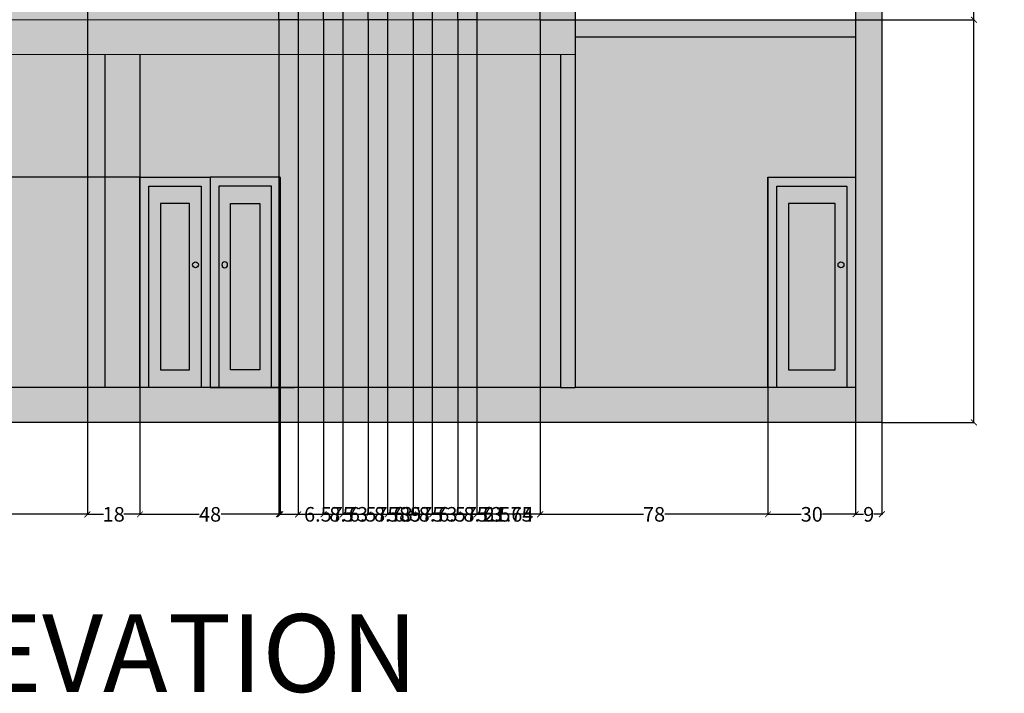
# Model space of a CAD drawing. Units: inches. Extents: x 1455 to 5994, y -182 to 2370.
# Tile 6 of 8: x 4579 to 4916, y -182 to 49. Entities that reach past the tile are written whole.
import ezdxf

# ---------------------------------------------------------------- set-up
doc = ezdxf.new("R2010")
doc.units = ezdxf.units.IN
doc.header["$MEASUREMENT"] = 0
doc.linetypes.add('CENTER', pattern=[50.8, 31.75, -6.35, 6.35, -6.35])
for name, color, linetype, lineweight in [('A-ANNO-DIMS', 2, 'Continuous', 18), ('A-ANNO-TEXT', 7, 'Continuous', 25), ('A-ELEV', 7, 'Continuous', 25), ('A-ELEV-PATT', 8, 'Continuous', 13), ('A-GRID', 8, 'CENTER', 18)]:
    doc.layers.add(name, color=color, linetype=linetype, lineweight=lineweight)
doc.styles.get("Standard").update_dxf_attribs({"font": 'arial.ttf'})
doc.dimstyles.get("Standard").update_dxf_attribs({"dimtxt": 5, "dimasz": 2, "dimexe": 0.18, "dimexo": 0.0625, "dimgap": 0.09, "dimtad": 0, "dimtih": 1, "dimtoh": 1, "dimdec": 1, "dimzin": 0, "dimdsep": 46, "dimlunit": 3, "dimtxsty": 'Standard', "dimblk": 'ARCHTICK', "dimcen": 0.09, "dimadec": 0, "dimazin": 0, "dimtfac": 1, "dimtdec": 1, "dimtofl": 0, "dimtmove": 0, "dimatfit": 3, "dimfxl": 1, "dimtolj": 1, "dimtzin": 0, "dimarcsym": 0})

# ---------------------------------------------------------------- blocks, each defined once
blk = doc.blocks.new('*U11')
blk.add_lwpolyline([(3.12, 0.01), (0.12, 0.01), (0.12, 72.01), (24.12, 72.01), (24.12, 0.01), (21.12, 0.01)])
for points in [[(21.12, 68.99), (21.12, 0.01), (3.12, 0.01), (3.12, 68.99)], [(17.12, 6.01), (17.12, 62.99), (7.12, 62.99), (7.12, 6.01)]]:
    blk.add_lwpolyline(points, close=True)
blk.add_circle((19.12, 42.01), 1)
blk = doc.blocks.new('*U12')
blk.add_lwpolyline([(3.12, 0.01), (0.12, 0.01), (0.12, 72.01), (30.12, 72.01), (30.12, 0.01), (27.12, 0.01)])
for points in [[(27.12, 68.99), (27.12, 0.01), (3.12, 0.01), (3.12, 68.99)], [(23.12, 6.01), (23.12, 62.99), (7.12, 62.99), (7.12, 6.01)]]:
    blk.add_lwpolyline(points, close=True)
blk.add_circle((25.12, 42.01), 1)
blk = doc.blocks.new('_ArchTick')
at = {"color": 0, "linetype": 'ByBlock', "const_width": 0.15}
blk.add_lwpolyline([(-0.5, -0.5), (0.5, 0.5)], dxfattribs=at)
blk = doc.blocks.new('*D84')
at = {"layer": 'A-ANNO-DIMS', "color": 0, "lineweight": -2, "transparency": 16777216}
for p, q in [((4873.75, 205.1), (4905.37, 205.1)), ((4905.19, 205.1), (4905.19, 60.74)), ((4905.19, -88.9), (4905.19, 55.45)), ((4873.75, -88.9), (4905.37, -88.9))]:
    blk.add_line(p, q, dxfattribs=at)
at = {"layer": 'Defpoints', "color": 0, "lineweight": 25, "transparency": 16777216}
for p in [(4873.69, 205.1), (4905.19, 205.1), (4873.69, -88.9)]:
    blk.add_point(p, dxfattribs=at)
at = {"layer": 'A-ANNO-DIMS', "color": 0, "lineweight": -2, "transparency": 16777216, "xscale": 2, "yscale": 2, "zscale": 2}
for p, rotation in [((4905.19, 205.1), 90), ((4905.19, -88.9), 270)]:
    blk.add_blockref('_ArchTick', p, dxfattribs=dict(at, rotation=rotation))
at = {"layer": 'A-ANNO-DIMS', "color": 0, "transparency": 16777216, "insert": (4905.19, 58.1), "char_height": 5, "attachment_point": 5}
blk.add_mtext('\\A1;294', dxfattribs=at)
blk = doc.blocks.new('*D89')
at = {"layer": 'A-ANNO-DIMS', "color": 0, "lineweight": -2, "transparency": 16777216}
for p, q in [((4396.19, 81.03), (4396.19, -120.58)), ((4601.69, 81.03), (4601.69, -120.58)), ((4396.19, -120.4), (4490.35, -120.4)), ((4601.69, -120.4), (4507.53, -120.4))]:
    blk.add_line(p, q, dxfattribs=at)
at = {"layer": 'Defpoints', "color": 0, "lineweight": 25, "transparency": 16777216}
for p in [(4396.19, 81.1), (4601.69, 81.1), (4601.69, -120.4)]:
    blk.add_point(p, dxfattribs=at)
at = {"layer": 'A-ANNO-DIMS', "color": 0, "lineweight": -2, "transparency": 16777216, "xscale": 2, "yscale": 2, "zscale": 2, "rotation": 180}
blk.add_blockref('_ArchTick', (4396.19, -120.4), dxfattribs=at)
at = {"layer": 'A-ANNO-DIMS', "color": 0, "lineweight": -2, "transparency": 16777216, "xscale": 2, "yscale": 2, "zscale": 2}
blk.add_blockref('_ArchTick', (4601.69, -120.4), dxfattribs=at)
at = {"layer": 'A-ANNO-DIMS', "color": 0, "transparency": 16777216, "insert": (4498.94, -120.4), "char_height": 5, "attachment_point": 5}
blk.add_mtext('\\A1;205.5', dxfattribs=at)
blk = doc.blocks.new('*D90')
at = {"layer": 'A-ANNO-DIMS', "color": 0, "lineweight": -2, "transparency": 16777216}
for p, q in [((4601.69, 81.03), (4601.69, -120.58)), ((4619.69, -4.97), (4619.69, -120.58)), ((4601.69, -120.4), (4607.25, -120.4)), ((4619.69, -120.4), (4614.13, -120.4))]:
    blk.add_line(p, q, dxfattribs=at)
at = {"layer": 'Defpoints', "color": 0, "lineweight": 25, "transparency": 16777216}
for p in [(4601.69, 81.1), (4619.69, -4.9), (4619.69, -120.4)]:
    blk.add_point(p, dxfattribs=at)
at = {"layer": 'A-ANNO-DIMS', "color": 0, "lineweight": -2, "transparency": 16777216, "xscale": 2, "yscale": 2, "zscale": 2, "rotation": 180}
blk.add_blockref('_ArchTick', (4601.69, -120.4), dxfattribs=at)
at = {"layer": 'A-ANNO-DIMS', "color": 0, "lineweight": -2, "transparency": 16777216, "xscale": 2, "yscale": 2, "zscale": 2}
blk.add_blockref('_ArchTick', (4619.69, -120.4), dxfattribs=at)
at = {"layer": 'A-ANNO-DIMS', "color": 0, "transparency": 16777216, "insert": (4610.69, -120.4), "char_height": 5, "attachment_point": 5}
blk.add_mtext('\\A1;18', dxfattribs=at)
blk = doc.blocks.new('*D91')
at = {"layer": 'A-ANNO-DIMS', "color": 0, "lineweight": -2, "transparency": 16777216}
for p, q in [((4619.69, -4.97), (4619.69, -120.58)), ((4667.69, -4.97), (4667.69, -120.58)), ((4619.69, -120.4), (4639.91, -120.4)), ((4667.69, -120.4), (4647.47, -120.4))]:
    blk.add_line(p, q, dxfattribs=at)
at = {"layer": 'Defpoints', "color": 0, "lineweight": 25, "transparency": 16777216}
for p in [(4619.69, -4.9), (4667.69, -4.9), (4667.69, -120.4)]:
    blk.add_point(p, dxfattribs=at)
at = {"layer": 'A-ANNO-DIMS', "color": 0, "lineweight": -2, "transparency": 16777216, "xscale": 2, "yscale": 2, "zscale": 2, "rotation": 180}
blk.add_blockref('_ArchTick', (4619.69, -120.4), dxfattribs=at)
at = {"layer": 'A-ANNO-DIMS', "color": 0, "lineweight": -2, "transparency": 16777216, "xscale": 2, "yscale": 2, "zscale": 2}
blk.add_blockref('_ArchTick', (4667.69, -120.4), dxfattribs=at)
at = {"layer": 'A-ANNO-DIMS', "color": 0, "transparency": 16777216, "insert": (4643.69, -120.4), "char_height": 5, "attachment_point": 5}
blk.add_mtext('\\A1;48', dxfattribs=at)
blk = doc.blocks.new('*D92')
at = {"layer": 'A-ANNO-DIMS', "color": 0, "lineweight": -2, "transparency": 16777216}
for p, q in [((4756.69, 48.95), (4756.69, -120.58)), ((4667.69, -4.97), (4667.69, -120.58)), ((4667.69, -120.4), (4708.51, -120.4)), ((4756.69, -120.4), (4715.87, -120.4))]:
    blk.add_line(p, q, dxfattribs=at)
at = {"layer": 'Defpoints', "color": 0, "lineweight": 25, "transparency": 16777216}
for p in [(4756.69, 49.01), (4667.69, -4.9), (4756.69, -120.4)]:
    blk.add_point(p, dxfattribs=at)
at = {"layer": 'A-ANNO-DIMS', "color": 0, "lineweight": -2, "transparency": 16777216, "xscale": 2, "yscale": 2, "zscale": 2, "rotation": 180}
blk.add_blockref('_ArchTick', (4667.69, -120.4), dxfattribs=at)
at = {"layer": 'A-ANNO-DIMS', "color": 0, "lineweight": -2, "transparency": 16777216, "xscale": 2, "yscale": 2, "zscale": 2}
blk.add_blockref('_ArchTick', (4756.69, -120.4), dxfattribs=at)
at = {"layer": 'A-ANNO-DIMS', "color": 0, "transparency": 16777216, "insert": (4712.19, -120.4), "char_height": 5, "attachment_point": 5}
blk.add_mtext('\\A1;89', dxfattribs=at)
blk = doc.blocks.new('*D93')
at = {"layer": 'A-ANNO-DIMS', "color": 0, "lineweight": -2, "transparency": 16777216}
for p, q in [((4756.69, 48.95), (4756.69, -120.58)), ((4834.69, -4.97), (4834.69, -120.58)), ((4756.69, -120.4), (4792.03, -120.4)), ((4834.69, -120.4), (4799.34, -120.4))]:
    blk.add_line(p, q, dxfattribs=at)
at = {"layer": 'Defpoints', "color": 0, "lineweight": 25, "transparency": 16777216}
for p in [(4756.69, 49.01), (4834.69, -4.9), (4834.69, -120.4)]:
    blk.add_point(p, dxfattribs=at)
at = {"layer": 'A-ANNO-DIMS', "color": 0, "lineweight": -2, "transparency": 16777216, "xscale": 2, "yscale": 2, "zscale": 2, "rotation": 180}
blk.add_blockref('_ArchTick', (4756.69, -120.4), dxfattribs=at)
at = {"layer": 'A-ANNO-DIMS', "color": 0, "lineweight": -2, "transparency": 16777216, "xscale": 2, "yscale": 2, "zscale": 2}
blk.add_blockref('_ArchTick', (4834.69, -120.4), dxfattribs=at)
at = {"layer": 'A-ANNO-DIMS', "color": 0, "transparency": 16777216, "insert": (4795.69, -120.4), "char_height": 5, "attachment_point": 5}
blk.add_mtext('\\A1;78', dxfattribs=at)
blk = doc.blocks.new('*D94')
at = {"layer": 'A-ANNO-DIMS', "color": 0, "lineweight": -2, "transparency": 16777216}
for p, q in [((4834.69, -4.97), (4834.69, -120.58)), ((4864.69, -4.97), (4864.69, -120.58)), ((4834.69, -120.4), (4846.03, -120.4)), ((4864.69, -120.4), (4853.35, -120.4))]:
    blk.add_line(p, q, dxfattribs=at)
at = {"layer": 'Defpoints', "color": 0, "lineweight": 25, "transparency": 16777216}
for p in [(4834.69, -4.9), (4864.69, -4.9), (4864.69, -120.4)]:
    blk.add_point(p, dxfattribs=at)
at = {"layer": 'A-ANNO-DIMS', "color": 0, "lineweight": -2, "transparency": 16777216, "xscale": 2, "yscale": 2, "zscale": 2, "rotation": 180}
blk.add_blockref('_ArchTick', (4834.69, -120.4), dxfattribs=at)
at = {"layer": 'A-ANNO-DIMS', "color": 0, "lineweight": -2, "transparency": 16777216, "xscale": 2, "yscale": 2, "zscale": 2}
blk.add_blockref('_ArchTick', (4864.69, -120.4), dxfattribs=at)
at = {"layer": 'A-ANNO-DIMS', "color": 0, "transparency": 16777216, "insert": (4849.69, -120.4), "char_height": 5, "attachment_point": 5}
blk.add_mtext('\\A1;30', dxfattribs=at)
blk = doc.blocks.new('*D95')
at = {"layer": 'A-ANNO-DIMS', "color": 0, "lineweight": -2, "transparency": 16777216}
for p, q in [((4864.69, -4.97), (4864.69, -120.58)), ((4873.69, -88.97), (4873.69, -120.58)), ((4864.69, -120.4), (4867.45, -120.4)), ((4873.69, -120.4), (4870.92, -120.4))]:
    blk.add_line(p, q, dxfattribs=at)
at = {"layer": 'Defpoints', "color": 0, "lineweight": 25, "transparency": 16777216}
for p in [(4864.69, -4.9), (4873.69, -88.9), (4873.69, -120.4)]:
    blk.add_point(p, dxfattribs=at)
at = {"layer": 'A-ANNO-DIMS', "color": 0, "lineweight": -2, "transparency": 16777216, "xscale": 2, "yscale": 2, "zscale": 2, "rotation": 180}
blk.add_blockref('_ArchTick', (4864.69, -120.4), dxfattribs=at)
at = {"layer": 'A-ANNO-DIMS', "color": 0, "lineweight": -2, "transparency": 16777216, "xscale": 2, "yscale": 2, "zscale": 2}
blk.add_blockref('_ArchTick', (4873.69, -120.4), dxfattribs=at)
at = {"layer": 'A-ANNO-DIMS', "color": 0, "transparency": 16777216, "insert": (4869.19, -120.4), "char_height": 5, "attachment_point": 5}
blk.add_mtext('\\A1;9', dxfattribs=at)
blk = doc.blocks.new('*D98')
at = {"layer": 'A-ANNO-DIMS', "color": 0, "lineweight": -2, "transparency": 16777216}
for p, q in [((4619.63, -4.9), (4245.01, -4.9)), ((4245.19, -4.9), (4245.19, -22.26)), ((4245.19, -44.9), (4245.19, -27.55)), ((4325.63, -44.9), (4245.01, -44.9))]:
    blk.add_line(p, q, dxfattribs=at)
at = {"layer": 'Defpoints', "color": 0, "lineweight": 25, "transparency": 16777216}
for p in [(4245.19, -4.9), (4619.69, -4.9), (4325.69, -44.9)]:
    blk.add_point(p, dxfattribs=at)
at = {"layer": 'A-ANNO-DIMS', "color": 0, "lineweight": -2, "transparency": 16777216, "xscale": 2, "yscale": 2, "zscale": 2}
for p, rotation in [((4245.19, -4.9), 90), ((4245.19, -44.9), 270)]:
    blk.add_blockref('_ArchTick', p, dxfattribs=dict(at, rotation=rotation))
at = {"layer": 'A-ANNO-DIMS', "color": 0, "transparency": 16777216, "insert": (4245.19, -24.9), "char_height": 5, "attachment_point": 5}
blk.add_mtext('\\A1;40', dxfattribs=at)
blk = doc.blocks.new('*D99')
at = {"layer": 'A-ANNO-DIMS', "color": 0, "lineweight": -2, "transparency": 16777216}
for p, q in [((4325.63, 11.1), (4245.01, 11.1)), ((4245.19, 11.1), (4245.19, 5.74)), ((4245.19, -4.9), (4245.19, 0.45)), ((4619.63, -4.9), (4245.01, -4.9))]:
    blk.add_line(p, q, dxfattribs=at)
at = {"layer": 'Defpoints', "color": 0, "lineweight": 25, "transparency": 16777216}
for p in [(4245.19, 11.1), (4325.69, 11.1), (4619.69, -4.9)]:
    blk.add_point(p, dxfattribs=at)
at = {"layer": 'A-ANNO-DIMS', "color": 0, "lineweight": -2, "transparency": 16777216, "xscale": 2, "yscale": 2, "zscale": 2}
for p, rotation in [((4245.19, 11.1), 90), ((4245.19, -4.9), 270)]:
    blk.add_blockref('_ArchTick', p, dxfattribs=dict(at, rotation=rotation))
at = {"layer": 'A-ANNO-DIMS', "color": 0, "transparency": 16777216, "insert": (4245.19, 3.1), "char_height": 5, "attachment_point": 5}
blk.add_mtext('\\A1;16', dxfattribs=at)
blk = doc.blocks.new('*D106')
at = {"layer": 'A-ANNO-DIMS', "color": 0, "lineweight": -2, "transparency": 16777216}
for p, q in [((4667.25, 48.96), (4667.25, -120.58)), ((4673.83, 48.96), (4673.83, -120.58)), ((4667.25, -120.4), (4673.83, -120.4)), ((4673.83, -120.4), (4675.83, -120.4))]:
    blk.add_line(p, q, dxfattribs=at)
at = {"layer": 'Defpoints', "color": 0, "lineweight": 25, "transparency": 16777216}
for p in [(4667.25, 49.03), (4673.83, 49.03), (4673.83, -120.4)]:
    blk.add_point(p, dxfattribs=at)
at = {"layer": 'A-ANNO-DIMS', "color": 0, "lineweight": -2, "transparency": 16777216, "xscale": 2, "yscale": 2, "zscale": 2, "rotation": 180}
blk.add_blockref('_ArchTick', (4667.25, -120.4), dxfattribs=at)
at = {"layer": 'A-ANNO-DIMS', "color": 0, "lineweight": -2, "transparency": 16777216, "xscale": 2, "yscale": 2, "zscale": 2}
blk.add_blockref('_ArchTick', (4673.83, -120.4), dxfattribs=at)
at = {"layer": 'A-ANNO-DIMS', "color": 0, "transparency": 16777216, "insert": (4684.38, -120.4), "char_height": 5, "attachment_point": 5}
blk.add_mtext('\\A1;6.575', dxfattribs=at)
blk = doc.blocks.new('*D107')
at = {"layer": 'A-ANNO-DIMS', "color": 0, "lineweight": -2, "transparency": 16777216}
for p, q in [((4673.83, 48.96), (4673.83, -120.58)), ((4682.56, 48.96), (4682.56, -120.58)), ((4673.83, -120.4), (4682.56, -120.4)), ((4682.56, -120.4), (4684.56, -120.4))]:
    blk.add_line(p, q, dxfattribs=at)
at = {"layer": 'Defpoints', "color": 0, "lineweight": 25, "transparency": 16777216}
for p in [(4673.83, 49.03), (4682.56, 49.03), (4682.56, -120.4)]:
    blk.add_point(p, dxfattribs=at)
at = {"layer": 'A-ANNO-DIMS', "color": 0, "lineweight": -2, "transparency": 16777216, "xscale": 2, "yscale": 2, "zscale": 2, "rotation": 180}
blk.add_blockref('_ArchTick', (4673.83, -120.4), dxfattribs=at)
at = {"layer": 'A-ANNO-DIMS', "color": 0, "lineweight": -2, "transparency": 16777216, "xscale": 2, "yscale": 2, "zscale": 2}
blk.add_blockref('_ArchTick', (4682.56, -120.4), dxfattribs=at)
at = {"layer": 'A-ANNO-DIMS', "color": 0, "transparency": 16777216, "insert": (4691.14, -120.4), "char_height": 5, "attachment_point": 5}
blk.add_mtext('\\A1;8.73', dxfattribs=at)
blk = doc.blocks.new('*D108')
at = {"layer": 'A-ANNO-DIMS', "color": 0, "lineweight": -2, "transparency": 16777216}
for p, q in [((4682.56, 48.96), (4682.56, -120.58)), ((4689.13, 48.96), (4689.13, -120.58)), ((4682.56, -120.4), (4689.13, -120.4)), ((4689.13, -120.4), (4691.13, -120.4))]:
    blk.add_line(p, q, dxfattribs=at)
at = {"layer": 'Defpoints', "color": 0, "lineweight": 25, "transparency": 16777216}
for p in [(4682.56, 49.03), (4689.13, 49.03), (4689.13, -120.4)]:
    blk.add_point(p, dxfattribs=at)
at = {"layer": 'A-ANNO-DIMS', "color": 0, "lineweight": -2, "transparency": 16777216, "xscale": 2, "yscale": 2, "zscale": 2, "rotation": 180}
blk.add_blockref('_ArchTick', (4682.56, -120.4), dxfattribs=at)
at = {"layer": 'A-ANNO-DIMS', "color": 0, "lineweight": -2, "transparency": 16777216, "xscale": 2, "yscale": 2, "zscale": 2}
blk.add_blockref('_ArchTick', (4689.13, -120.4), dxfattribs=at)
at = {"layer": 'A-ANNO-DIMS', "color": 0, "transparency": 16777216, "insert": (4699.69, -120.4), "char_height": 5, "attachment_point": 5}
blk.add_mtext('\\A1;6.575', dxfattribs=at)
blk = doc.blocks.new('*D109')
at = {"layer": 'A-ANNO-DIMS', "color": 0, "lineweight": -2, "transparency": 16777216}
for p, q in [((4689.13, 48.96), (4689.13, -120.58)), ((4697.86, 48.96), (4697.86, -120.58)), ((4689.13, -120.4), (4697.86, -120.4)), ((4697.86, -120.4), (4699.86, -120.4))]:
    blk.add_line(p, q, dxfattribs=at)
at = {"layer": 'Defpoints', "color": 0, "lineweight": 25, "transparency": 16777216}
for p in [(4689.13, 49.03), (4697.86, 49.03), (4697.86, -120.4)]:
    blk.add_point(p, dxfattribs=at)
at = {"layer": 'A-ANNO-DIMS', "color": 0, "lineweight": -2, "transparency": 16777216, "xscale": 2, "yscale": 2, "zscale": 2, "rotation": 180}
blk.add_blockref('_ArchTick', (4689.13, -120.4), dxfattribs=at)
at = {"layer": 'A-ANNO-DIMS', "color": 0, "lineweight": -2, "transparency": 16777216, "xscale": 2, "yscale": 2, "zscale": 2}
blk.add_blockref('_ArchTick', (4697.86, -120.4), dxfattribs=at)
at = {"layer": 'A-ANNO-DIMS', "color": 0, "transparency": 16777216, "insert": (4706.45, -120.4), "char_height": 5, "attachment_point": 5}
blk.add_mtext('\\A1;8.73', dxfattribs=at)
blk = doc.blocks.new('*D110')
at = {"layer": 'A-ANNO-DIMS', "color": 0, "lineweight": -2, "transparency": 16777216}
for p, q in [((4697.86, 48.96), (4697.86, -120.58)), ((4704.44, 48.96), (4704.44, -120.58)), ((4697.86, -120.4), (4704.44, -120.4)), ((4704.44, -120.4), (4706.44, -120.4))]:
    blk.add_line(p, q, dxfattribs=at)
at = {"layer": 'Defpoints', "color": 0, "lineweight": 25, "transparency": 16777216}
for p in [(4697.86, 49.03), (4704.44, 49.03), (4704.44, -120.4)]:
    blk.add_point(p, dxfattribs=at)
at = {"layer": 'A-ANNO-DIMS', "color": 0, "lineweight": -2, "transparency": 16777216, "xscale": 2, "yscale": 2, "zscale": 2, "rotation": 180}
blk.add_blockref('_ArchTick', (4697.86, -120.4), dxfattribs=at)
at = {"layer": 'A-ANNO-DIMS', "color": 0, "lineweight": -2, "transparency": 16777216, "xscale": 2, "yscale": 2, "zscale": 2}
blk.add_blockref('_ArchTick', (4704.44, -120.4), dxfattribs=at)
at = {"layer": 'A-ANNO-DIMS', "color": 0, "transparency": 16777216, "insert": (4715, -120.4), "char_height": 5, "attachment_point": 5}
blk.add_mtext('\\A1;6.575', dxfattribs=at)
blk = doc.blocks.new('*D111')
at = {"layer": 'A-ANNO-DIMS', "color": 0, "lineweight": -2, "transparency": 16777216}
for p, q in [((4704.44, 48.96), (4704.44, -120.58)), ((4713.17, 48.96), (4713.17, -120.58)), ((4704.44, -120.4), (4713.17, -120.4)), ((4713.17, -120.4), (4715.17, -120.4))]:
    blk.add_line(p, q, dxfattribs=at)
at = {"layer": 'Defpoints', "color": 0, "lineweight": 25, "transparency": 16777216}
for p in [(4704.44, 49.03), (4713.17, 49.03), (4713.17, -120.4)]:
    blk.add_point(p, dxfattribs=at)
at = {"layer": 'A-ANNO-DIMS', "color": 0, "lineweight": -2, "transparency": 16777216, "xscale": 2, "yscale": 2, "zscale": 2, "rotation": 180}
blk.add_blockref('_ArchTick', (4704.44, -120.4), dxfattribs=at)
at = {"layer": 'A-ANNO-DIMS', "color": 0, "lineweight": -2, "transparency": 16777216, "xscale": 2, "yscale": 2, "zscale": 2}
blk.add_blockref('_ArchTick', (4713.17, -120.4), dxfattribs=at)
at = {"layer": 'A-ANNO-DIMS', "color": 0, "transparency": 16777216, "insert": (4721.75, -120.4), "char_height": 5, "attachment_point": 5}
blk.add_mtext('\\A1;8.73', dxfattribs=at)
blk = doc.blocks.new('*D112')
at = {"layer": 'A-ANNO-DIMS', "color": 0, "lineweight": -2, "transparency": 16777216}
for p, q in [((4713.17, 48.96), (4713.17, -120.58)), ((4719.74, 48.96), (4719.74, -120.58)), ((4713.17, -120.4), (4719.74, -120.4)), ((4719.74, -120.4), (4721.74, -120.4))]:
    blk.add_line(p, q, dxfattribs=at)
at = {"layer": 'Defpoints', "color": 0, "lineweight": 25, "transparency": 16777216}
for p in [(4713.17, 49.03), (4719.74, 49.03), (4719.74, -120.4)]:
    blk.add_point(p, dxfattribs=at)
at = {"layer": 'A-ANNO-DIMS', "color": 0, "lineweight": -2, "transparency": 16777216, "xscale": 2, "yscale": 2, "zscale": 2, "rotation": 180}
blk.add_blockref('_ArchTick', (4713.17, -120.4), dxfattribs=at)
at = {"layer": 'A-ANNO-DIMS', "color": 0, "lineweight": -2, "transparency": 16777216, "xscale": 2, "yscale": 2, "zscale": 2}
blk.add_blockref('_ArchTick', (4719.74, -120.4), dxfattribs=at)
at = {"layer": 'A-ANNO-DIMS', "color": 0, "transparency": 16777216, "insert": (4730.3, -120.4), "char_height": 5, "attachment_point": 5}
blk.add_mtext('\\A1;6.575', dxfattribs=at)
blk = doc.blocks.new('*D113')
at = {"layer": 'A-ANNO-DIMS', "color": 0, "lineweight": -2, "transparency": 16777216}
for p, q in [((4719.74, 48.96), (4719.74, -120.58)), ((4728.47, 48.96), (4728.47, -120.58)), ((4719.74, -120.4), (4728.47, -120.4)), ((4728.47, -120.4), (4730.47, -120.4))]:
    blk.add_line(p, q, dxfattribs=at)
at = {"layer": 'Defpoints', "color": 0, "lineweight": 25, "transparency": 16777216}
for p in [(4719.74, 49.03), (4728.47, 49.03), (4728.47, -120.4)]:
    blk.add_point(p, dxfattribs=at)
at = {"layer": 'A-ANNO-DIMS', "color": 0, "lineweight": -2, "transparency": 16777216, "xscale": 2, "yscale": 2, "zscale": 2, "rotation": 180}
blk.add_blockref('_ArchTick', (4719.74, -120.4), dxfattribs=at)
at = {"layer": 'A-ANNO-DIMS', "color": 0, "lineweight": -2, "transparency": 16777216, "xscale": 2, "yscale": 2, "zscale": 2}
blk.add_blockref('_ArchTick', (4728.47, -120.4), dxfattribs=at)
at = {"layer": 'A-ANNO-DIMS', "color": 0, "transparency": 16777216, "insert": (4737.06, -120.4), "char_height": 5, "attachment_point": 5}
blk.add_mtext('\\A1;8.73', dxfattribs=at)
blk = doc.blocks.new('*D114')
at = {"layer": 'A-ANNO-DIMS', "color": 0, "lineweight": -2, "transparency": 16777216}
for p, q in [((4728.47, 48.96), (4728.47, -120.58)), ((4735.05, 48.96), (4735.05, -120.58)), ((4728.47, -120.4), (4735.05, -120.4)), ((4735.05, -120.4), (4737.05, -120.4))]:
    blk.add_line(p, q, dxfattribs=at)
at = {"layer": 'Defpoints', "color": 0, "lineweight": 25, "transparency": 16777216}
for p in [(4728.47, 49.03), (4735.05, 49.03), (4735.05, -120.4)]:
    blk.add_point(p, dxfattribs=at)
at = {"layer": 'A-ANNO-DIMS', "color": 0, "lineweight": -2, "transparency": 16777216, "xscale": 2, "yscale": 2, "zscale": 2, "rotation": 180}
blk.add_blockref('_ArchTick', (4728.47, -120.4), dxfattribs=at)
at = {"layer": 'A-ANNO-DIMS', "color": 0, "lineweight": -2, "transparency": 16777216, "xscale": 2, "yscale": 2, "zscale": 2}
blk.add_blockref('_ArchTick', (4735.05, -120.4), dxfattribs=at)
at = {"layer": 'A-ANNO-DIMS', "color": 0, "transparency": 16777216, "insert": (4745.61, -120.4), "char_height": 5, "attachment_point": 5}
blk.add_mtext('\\A1;6.575', dxfattribs=at)
blk = doc.blocks.new('*D115')
at = {"layer": 'A-ANNO-DIMS', "color": 0, "lineweight": -2, "transparency": 16777216}
for p, q in [((4735.05, 48.96), (4735.05, -120.58)), ((4756.69, 48.95), (4756.69, -120.58)), ((4735.05, -120.4), (4737.31, -120.4)), ((4756.69, -120.4), (4754.43, -120.4))]:
    blk.add_line(p, q, dxfattribs=at)
at = {"layer": 'Defpoints', "color": 0, "lineweight": 25, "transparency": 16777216}
for p in [(4735.05, 49.03), (4756.69, 49.01), (4756.69, -120.4)]:
    blk.add_point(p, dxfattribs=at)
at = {"layer": 'A-ANNO-DIMS', "color": 0, "lineweight": -2, "transparency": 16777216, "xscale": 2, "yscale": 2, "zscale": 2, "rotation": 180}
blk.add_blockref('_ArchTick', (4735.05, -120.4), dxfattribs=at)
at = {"layer": 'A-ANNO-DIMS', "color": 0, "lineweight": -2, "transparency": 16777216, "xscale": 2, "yscale": 2, "zscale": 2}
blk.add_blockref('_ArchTick', (4756.69, -120.4), dxfattribs=at)
at = {"layer": 'A-ANNO-DIMS', "color": 0, "transparency": 16777216, "insert": (4745.87, -120.4), "char_height": 5, "attachment_point": 5}
blk.add_mtext('\\A1;21.64', dxfattribs=at)
blk = doc.blocks.new('*D116')
at = {"layer": 'A-ANNO-DIMS', "color": 0, "lineweight": -2, "transparency": 16777216}
for p, q in [((4756.75, 157.1), (4905.37, 157.1)), ((4905.19, 157.1), (4905.19, 105.7)), ((4905.19, 49.01), (4905.19, 100.41)), ((4756.75, 49.01), (4905.37, 49.01))]:
    blk.add_line(p, q, dxfattribs=at)
at = {"layer": 'Defpoints', "color": 0, "lineweight": 25, "transparency": 16777216}
for p in [(4756.69, 157.1), (4905.19, 157.1), (4756.69, 49.01)]:
    blk.add_point(p, dxfattribs=at)
at = {"layer": 'A-ANNO-DIMS', "color": 0, "lineweight": -2, "transparency": 16777216, "xscale": 2, "yscale": 2, "zscale": 2}
for p, rotation in [((4905.19, 157.1), 90), ((4905.19, 49.01), 270)]:
    blk.add_blockref('_ArchTick', p, dxfattribs=dict(at, rotation=rotation))
at = {"layer": 'A-ANNO-DIMS', "color": 0, "transparency": 16777216, "insert": (4905.19, 103.06), "char_height": 5, "attachment_point": 5}
blk.add_mtext('\\A1;108.08', dxfattribs=at)

msp = doc.modelspace()

# ---------------------------------------------------------------- hatches: boundary and pattern name
at = {"layer": 'A-ELEV-PATT', "transparency": 33554641}
h = msp.add_hatch(color=256, dxfattribs=at)
h.dxf.hatch_style = 1
h.paths.add_polyline_path([(4768.6884, 169.0969), (4284.6884, 169.0969), (4276.6884, 169.0969), (4276.6884, 157.0969), (4756.6884, 157.0969), (4756.6884, 49.0187), (4719.7422, 49.0288), (4719.7422, 49.0261), (4713.167, 49.0261), (4704.4367, 49.0287), (4704.4367, 49.0261), (4697.8615, 49.0261), (4689.1312, 49.0288), (4689.1312, 49.0261), (4682.556, 49.0261), (4673.8258, 49.029), (4673.8258, 49.0261), (4667.2505, 49.0261), (4471.4513, 49.0969), (4284.6884, 49.0969), (4276.6884, 49.0969), (4276.6884, 37.0915), (4543.7991, 37.0915), (4768.6843, 37.0146)])
h = msp.add_hatch(color=256, dxfattribs=at)
h.dxf.hatch_style = 1
h.paths.add_polyline_path([(4873.6884, 169.0969), (4864.6884, 169.0969), (4864.6884, 85.0969), (4864.6884, 49.0146), (4864.6884, 43.0969), (4864.6884, -70.9031), (4864.6884, -76.9031), (4861.6884, -76.9031), (4837.6884, -76.9031), (4834.6884, -76.9031), (4768.6884, -76.9031), (4763.6884, -76.9031), (4284.6884, -76.9031), (4284.6884, -88.9031), (4873.6884, -88.9031)])
h = msp.add_hatch(color=256, dxfattribs=at)
h.dxf.hatch_style = 1
h.paths.add_polyline_path([(4756.6884, 157.0969), (4735.0477, 157.0969), (4735.0477, 49.0246), (4756.6884, 49.0187)])
h.paths.add_polyline_path([(4728.4725, 157.0969), (4719.7422, 157.0969), (4719.7422, 49.0288), (4728.4725, 49.0264)])
h.paths.add_polyline_path([(4713.167, 157.0969), (4704.4367, 157.0969), (4704.4367, 49.033), (4713.167, 49.0306)])
h.paths.add_polyline_path([(4697.8615, 157.0969), (4689.1312, 157.0969), (4689.1312, 49.0372), (4697.8615, 49.0348)])
h.paths.add_polyline_path([(4682.556, 157.0969), (4673.8258, 157.0969), (4673.8258, 49.0414), (4682.556, 49.039)])
h.paths.add_polyline_path([(4864.6884, 169.0969), (4768.6884, 169.0969), (4768.6858, 85.0969), (4864.6884, 85.0969)])
h = msp.add_hatch(color=256, dxfattribs=at)
h.dxf.hatch_style = 1
h.paths.add_polyline_path([(4471.4513, 157.0969), (4284.6884, 157.0969), (4284.6884, 49.0969), (4471.4513, 49.0969), (4471.4513, 85.0969)])
h.paths.add_polyline_path([(4396.1884, 85.0969), (4396.1884, 81.0969), (4344.1884, 81.0969), (4340.1884, 81.0969), (4340.1884, 137.0969), (4344.1884, 137.0969), (4392.1884, 137.0969), (4396.1884, 137.0969)], flags=16)
h.paths.add_polyline_path([(4607.6884, 37.0697), (4543.7991, 37.0915), (4284.6884, 37.0915), (4284.6884, -76.9031), (4607.6884, -76.9031)])
h.paths.add_polyline_path([(4381.6884, -40.9031), (4381.6884, -44.9031), (4329.6884, -44.9031), (4325.6884, -44.9031), (4325.6884, 11.0969), (4329.6884, 11.0969), (4377.6884, 11.0969), (4381.6884, 11.0969)], flags=16)
h.paths.add_polyline_path([(4377.6884, -40.9031), (4329.6884, -40.9031), (4329.6884, 7.0969), (4377.6884, 7.0969)], flags=0)
h.paths.add_polyline_path([(4376.1884, -39.4031), (4353.6884, -39.4031), (4331.1884, -39.4031), (4331.1884, 5.5969), (4353.6884, 5.5969), (4376.1884, 5.5969)], flags=0)
h.paths.add_polyline_path([(4375.1884, -38.4031), (4353.6884, -38.4031), (4353.6884, 4.5969), (4375.1884, 4.5969)], flags=0)
h.paths.add_polyline_path([(4352.6884, -38.4031), (4332.1884, -38.4031), (4332.1884, 4.5969), (4352.6884, 4.5969)], flags=0)
h.paths.add_polyline_path([(4667.2505, 157.0969), (4543.8032, 157.0969), (4543.8032, 85.0969), (4543.8032, 49.0771), (4667.2505, 49.0432)])
h.paths.add_polyline_path([(4601.6884, 81.0969), (4601.6884, 137.0969), (4605.6884, 137.0969), (4653.6884, 137.0969), (4657.6884, 137.0969), (4657.6884, 81.0969)], flags=16)
h.paths.add_polyline_path([(4543.8032, 157.0969), (4471.4513, 157.0969), (4471.4513, 85.0969), (4543.8032, 85.0969)])
h.paths.add_polyline_path([(4763.6884, 37.0163), (4619.6884, 37.0656), (4619.6884, -4.9031), (4643.6884, -4.9031), (4667.6884, -4.9031), (4667.6884, -76.9031), (4763.6884, -76.9031)])
h.paths.add_polyline_path([(4864.6884, 43.0969), (4768.6884, 43.0969), (4768.6884, -76.9031), (4834.6884, -76.9031), (4834.6884, -4.9031), (4864.6884, -4.9031)])
h = msp.add_hatch(color=256, dxfattribs=at)
h.dxf.hatch_style = 1
h.paths.add_polyline_path([(4735.0477, 157.0969), (4728.4725, 157.0969), (4728.4725, 49.0283), (4735.0477, 49.0261)])
h.paths.add_polyline_path([(4719.7422, 157.0969), (4713.167, 157.0969), (4713.167, 49.0336), (4719.7422, 49.0313)])
h.paths.add_polyline_path([(4704.4367, 157.0969), (4697.8615, 157.0969), (4697.8615, 49.0388), (4704.4367, 49.0366)])
h.paths.add_polyline_path([(4689.1312, 157.0969), (4682.556, 157.0969), (4682.556, 49.0441), (4689.1312, 49.0418)])
h.paths.add_polyline_path([(4673.8258, 157.0969), (4667.2505, 157.0969), (4667.2505, 49.0493), (4673.8258, 49.047)])
h = msp.add_hatch(color=256, dxfattribs=at)
h.dxf.hatch_style = 1
h.paths.add_polyline_path([(4864.6884, 49.0146), (4768.6847, 49.0146), (4768.6845, 43.0969), (4864.6884, 43.0969)])
h = msp.add_hatch(color=256, dxfattribs=at)
h.dxf.hatch_style = 1
h.paths.add_polyline_path([(4619.6884, 37.0656), (4607.6884, 37.0697), (4607.6884, -76.9031), (4619.6884, -76.9031)])
h = msp.add_hatch(color=256, dxfattribs=at)
h.dxf.hatch_style = 1
h.paths.add_polyline_path([(4768.6884, 37.0146), (4763.6884, 37.0163), (4763.6884, -76.9031), (4768.6884, -76.9031)])
h = msp.add_hatch(color=256, dxfattribs=at)
h.dxf.hatch_style = 1
h.paths.add_polyline_path([(4664.6884, -7.9261), (4646.6884, -7.9261), (4646.6884, -76.9031), (4664.6884, -76.9031)], flags=17)
h.paths.add_polyline_path([(4660.6884, -13.9261), (4660.6884, -70.9031), (4650.6884, -70.9031), (4650.6884, -13.9261)], flags=0)
h.paths.add_polyline_path([(4649.6884, -34.9031, -1), (4647.6884, -34.9031, -1)], flags=16)
h.paths.add_polyline_path([(4643.6884, -4.9031), (4619.6884, -4.9031), (4619.6884, -76.9031), (4622.6884, -76.9031), (4622.6884, -7.9261), (4640.6884, -7.9261), (4640.6884, -76.9031), (4643.6884, -76.9031)])
h.paths.add_polyline_path([(4640.6884, -7.9261), (4622.6884, -7.9261), (4622.6884, -76.9031), (4640.6884, -76.9031)], flags=17)
h.paths.add_polyline_path([(4636.6884, -13.9261), (4636.6884, -70.9031), (4626.6884, -70.9031), (4626.6884, -13.9261)], flags=0)
h.paths.add_polyline_path([(4639.6884, -34.9031, -1), (4637.6884, -34.9031, -1)], flags=16)
h.paths.add_polyline_path([(4636.6884, -13.9261), (4626.6884, -13.9261), (4626.6884, -70.9031), (4636.6884, -70.9031)], flags=16)
h.paths.add_polyline_path([(4660.6884, -13.9261), (4650.6884, -13.9261), (4650.6884, -70.9031), (4660.6884, -70.9031)], flags=16)
h.paths.add_polyline_path([(4667.6884, -4.9031), (4643.6884, -4.9031), (4643.6884, -76.9031), (4646.6884, -76.9031), (4646.6884, -7.9261), (4664.6884, -7.9261), (4664.6884, -76.9031), (4667.6884, -76.9031)])
h = msp.add_hatch(color=256, dxfattribs=at)
h.dxf.hatch_style = 1
h.paths.add_polyline_path([(4660.6884, -13.9261), (4650.6884, -13.9261), (4650.6884, -70.9031), (4660.6884, -70.9031)])
h.paths.add_polyline_path([(4636.6884, -13.9261), (4626.6884, -13.9261), (4626.6884, -70.9031), (4636.6884, -70.9031)])
h.paths.add_polyline_path([(4857.6884, -13.9261), (4841.6884, -13.9261), (4841.6884, -70.9031), (4857.6884, -70.9031)], flags=0)
h.paths.add_polyline_path([(4861.6884, -7.9261), (4837.6884, -7.9261), (4837.6884, -76.9031), (4861.6884, -76.9031)], flags=17)
h.paths.add_polyline_path([(4857.6884, -13.9261), (4857.6884, -70.9031), (4841.6884, -70.9031), (4841.6884, -13.9261)], flags=16)
h.paths.add_polyline_path([(4860.6884, -34.9031, -1), (4858.6884, -34.9031, -1)], flags=16)
h.paths.add_polyline_path([(4864.6884, -4.9031), (4834.6884, -4.9031), (4834.6884, -76.9031), (4837.6884, -76.9031), (4837.6884, -7.9261), (4861.6884, -7.9261), (4861.6884, -76.9031), (4864.6884, -76.9031)])
h = msp.add_hatch(color=256, dxfattribs=at)
h.dxf.hatch_style = 1
h.paths.add_polyline_path([(4857.6884, -13.9261), (4841.6884, -13.9261), (4841.6884, -70.9031), (4857.6884, -70.9031)])
h = msp.add_hatch(color=256, dxfattribs=at)
h.dxf.hatch_style = 1
h.paths.add_polyline_path([(4647.6884, -34.9031, 1), (4649.6884, -34.9031, 1)])
h.paths.add_polyline_path([(4639.6884, -34.9031, 1), (4637.6884, -34.9031, 1)])
h.paths.add_polyline_path([(4860.6884, -34.9031, 1), (4858.6884, -34.9031, 1)])

# ---------------------------------------------------------------- linework, layer by layer
at = {"layer": 'A-ELEV'}
for p, q in [((4873.6884, 169.0969), (4873.6884, -88.9031)), ((4864.6884, 85.0969), (4864.6884, 49.0146)), ((4768.6884, 49.0146), (4864.6884, 49.0146)), ((4864.6884, 49.0146), (4864.6884, 43.0969)), ((4864.6884, 43.0969), (4768.6884, 43.0969)), ((4768.6884, 43.0969), (4768.6884, -76.9031)), ((4768.6884, 43.0969), (4768.6884, -76.9031)), ((4864.6884, 43.0969), (4864.6884, -70.9031)), ((4607.6884, 37.0697), (4607.6884, -76.9031)), ((4619.6884, 37.0656), (4619.6884, -76.9031)), ((4763.6884, 37.0163), (4763.6884, -76.9031)), ((4834.6884, -4.9031), (4834.6884, -76.9031)), ((4763.6884, -76.9031), (4284.6884, -76.9031)), ((4667.5607, -76.9158), (4672.5607, -76.9158)), ((4763.6884, -76.9031), (4768.6884, -76.9031)), ((4864.6884, -76.9031), (4768.6884, -76.9031)), ((4873.6884, -88.9031), (4284.6884, -88.9031))]:
    msp.add_line(p, q, dxfattribs=at)
msp.add_lwpolyline([(4756.6884, 49.0146), (4756.6884, 157.0969), (4276.6884, 157.0969), (4276.6884, 169.0969), (4284.6884, 169.0969), (4768.6884, 169.0969), (4768.6843, 37.0146), (4543.7991, 37.0915), (4276.6884, 37.0915), (4276.6884, 49.0969), (4284.6884, 49.0969), (4471.4513, 49.0969), (4756.6884, 49.0187)], dxfattribs=at)
for points in [[(4667.2505, 157.0969), (4673.8258, 157.0969), (4673.8258, 49.0261), (4667.2505, 49.0261)], [(4682.556, 157.0969), (4689.1312, 157.0969), (4689.1312, 49.0261), (4682.556, 49.0261)], [(4697.8615, 157.0969), (4704.4367, 157.0969), (4704.4367, 49.0261), (4697.8615, 49.0261)], [(4713.167, 157.0969), (4719.7422, 157.0969), (4719.7422, 49.0261), (4713.167, 49.0261)], [(4728.4725, 157.0969), (4735.0477, 157.0969), (4735.0477, 49.0261), (4728.4725, 49.0261)]]:
    msp.add_lwpolyline(points, close=True, dxfattribs=at)
at = {"layer": 'A-GRID'}
msp.add_line((4873.6884, 43.0969), (4873.6884, -88.9031), dxfattribs=at)

# ---------------------------------------------------------------- block references
at = {"layer": 'A-ELEV'}
for name, p in [('*U11', (4619.5647, -76.9158)), ('*U12', (4834.5647, -76.9158))]:
    msp.add_blockref(name, p, dxfattribs=at)
at = {"layer": 'A-ELEV', "xscale": -1}
msp.add_blockref('*U11', (4667.8122, -76.9158), dxfattribs=at)

# ---------------------------------------------------------------- texts
at = {"layer": 'A-ANNO-TEXT'}
msp.add_text('FRONT ELEVATION', height=26.640459, dxfattribs=at).set_placement((4397.2929, -181.252))

# ---------------------------------------------------------------- dimensions: what is measured, and where the dimension line sits
at = {"layer": 'A-ANNO-DIMS'}
for base, p1, p2, override, picture, middle in [((4905.1884, 205.0969), (4873.6884, -88.9031), (4873.6884, 205.0969), {"dimdec": 0, "dimlfac": 1, "dimrnd": 0, "dimzin": 0, "dimdsep": 46, "dimlunit": 2}, '*D84', (4905.1884, 58.0969)), ((4905.1884, 157.0969), (4756.6884, 49.0146), (4756.6884, 157.0969), {"dimdec": 2, "dimlfac": 1, "dimrnd": 0, "dimzin": 0, "dimdsep": 46, "dimlunit": 2}, '*D116', (4905.1884, 103.0558)), ((4245.1884, 11.0969), (4619.6884, -4.9031), (4325.6884, 11.0969), {"dimdec": 0, "dimlfac": 1, "dimrnd": 0, "dimzin": 0, "dimdsep": 46, "dimlunit": 2}, '*D99', (4245.1884, 3.0969)), ((4245.1884, -4.9031), (4325.6884, -44.9031), (4619.6884, -4.9031), {"dimdec": 0, "dimlfac": 1, "dimrnd": 0, "dimzin": 0, "dimdsep": 46, "dimlunit": 2}, '*D98', (4245.1884, -24.9031))]:
    dim = msp.add_linear_dim(base=base, p1=p1, p2=p2, angle=90, dimstyle='Standard', override=override, dxfattribs=at)
    dim.commit()
    dim.dimension.update_dxf_attribs({"geometry": picture, "text_midpoint": middle})
for base, p1, p2, override, picture, middle in [((4601.6884, -120.4031), (4396.1884, 81.0969), (4601.6884, 81.0969), {"dimdec": 1, "dimlfac": 1, "dimrnd": 0, "dimzin": 0, "dimdsep": 46, "dimlunit": 2}, '*D89', (4498.9384, -120.4031)), ((4619.6884, -120.4031), (4601.6884, 81.0969), (4619.6884, -4.9031), {"dimdec": 0, "dimlfac": 1, "dimrnd": 0, "dimzin": 0, "dimdsep": 46, "dimlunit": 2}, '*D90', (4610.6884, -120.4031)), ((4673.8258, -120.4031), (4667.2505, 49.0261), (4673.8258, 49.0261), {"dimdec": 3, "dimlfac": 1, "dimrnd": 0, "dimzin": 0, "dimdsep": 46, "dimlunit": 2}, '*D106', (4684.3844, -120.4031)), ((4756.6884, -120.4031), (4667.6884, -4.9031), (4756.6884, 49.0146), {"dimdec": 0, "dimlfac": 1, "dimrnd": 0, "dimzin": 0, "dimdsep": 46, "dimlunit": 2}, '*D92', (4712.1884, -120.4031)), ((4682.556, -120.4031), (4673.8258, 49.0261), (4682.556, 49.0261), {"dimdec": 2, "dimlfac": 1, "dimrnd": 0, "dimzin": 0, "dimdsep": 46, "dimlunit": 2}, '*D107', (4691.1433, -120.4031)), ((4689.1312, -120.4031), (4682.556, 49.0261), (4689.1312, 49.0261), {"dimdec": 3, "dimlfac": 1, "dimrnd": 0, "dimzin": 0, "dimdsep": 46, "dimlunit": 2}, '*D108', (4699.6899, -120.4031)), ((4697.8615, -120.4031), (4689.1312, 49.0261), (4697.8615, 49.0261), {"dimdec": 2, "dimlfac": 1, "dimrnd": 0, "dimzin": 0, "dimdsep": 46, "dimlunit": 2}, '*D109', (4706.4488, -120.4031)), ((4704.4367, -120.4031), (4697.8615, 49.0261), (4704.4367, 49.0261), {"dimdec": 3, "dimlfac": 1, "dimrnd": 0, "dimzin": 0, "dimdsep": 46, "dimlunit": 2}, '*D110', (4714.9954, -120.4031)), ((4713.167, -120.4031), (4704.4367, 49.0261), (4713.167, 49.0261), {"dimdec": 2, "dimlfac": 1, "dimrnd": 0, "dimzin": 0, "dimdsep": 46, "dimlunit": 2}, '*D111', (4721.7543, -120.4031)), ((4719.7422, -120.4031), (4713.167, 49.0261), (4719.7422, 49.0261), {"dimdec": 3, "dimlfac": 1, "dimrnd": 0, "dimzin": 0, "dimdsep": 46, "dimlunit": 2}, '*D112', (4730.3008, -120.4031)), ((4728.4725, -120.4031), (4719.7422, 49.0261), (4728.4725, 49.0261), {"dimdec": 2, "dimlfac": 1, "dimrnd": 0, "dimzin": 0, "dimdsep": 46, "dimlunit": 2}, '*D113', (4737.0597, -120.4031)), ((4735.0477, -120.4031), (4728.4725, 49.0261), (4735.0477, 49.0261), {"dimdec": 3, "dimlfac": 1, "dimrnd": 0, "dimzin": 0, "dimdsep": 46, "dimlunit": 2}, '*D114', (4745.6063, -120.4031)), ((4756.6884, -120.4031), (4735.0477, 49.0261), (4756.6884, 49.0146), {"dimdec": 2, "dimlfac": 1, "dimrnd": 0, "dimzin": 0, "dimdsep": 46, "dimlunit": 2}, '*D115', (4745.8681, -120.4031)), ((4834.6884, -120.4031), (4756.6884, 49.0146), (4834.6884, -4.9031), {"dimdec": 0, "dimlfac": 1, "dimrnd": 0, "dimzin": 0, "dimdsep": 46, "dimlunit": 2}, '*D93', (4795.6884, -120.4031)), ((4667.6884, -120.4031), (4619.6884, -4.9031), (4667.6884, -4.9031), {"dimdec": 0, "dimlfac": 1, "dimrnd": 0, "dimzin": 0, "dimdsep": 46, "dimlunit": 2}, '*D91', (4643.6884, -120.4031)), ((4864.6884, -120.4031), (4834.6884, -4.9031), (4864.6884, -4.9031), {"dimdec": 0, "dimlfac": 1, "dimrnd": 0, "dimzin": 0, "dimdsep": 46, "dimlunit": 2}, '*D94', (4849.6884, -120.4031)), ((4873.6884, -120.4031), (4864.6884, -4.9031), (4873.6884, -88.9031), {"dimdec": 0, "dimlfac": 1, "dimrnd": 0, "dimzin": 0, "dimdsep": 46, "dimlunit": 2}, '*D95', (4869.1884, -120.4031))]:
    dim = msp.add_linear_dim(base=base, p1=p1, p2=p2, dimstyle='Standard', override=override, dxfattribs=at)
    dim.commit()
    dim.dimension.update_dxf_attribs({"geometry": picture, "text_midpoint": middle})

doc.saveas('drawing.dxf')
